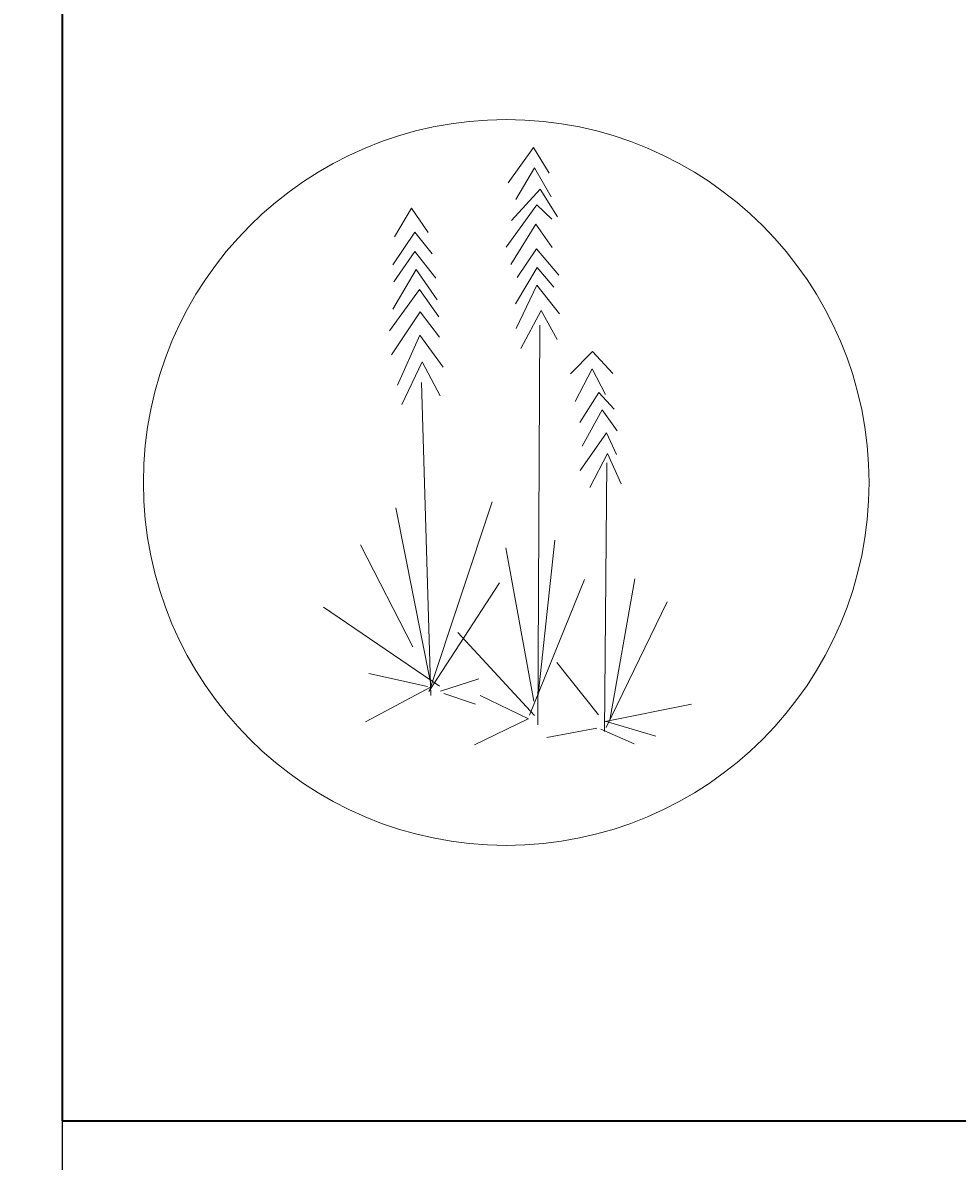
# Model space of a CAD drawing. Units: inches. Extents: x 8049 to 8459, y 820 to 1350.
# Tile 3 of 25: x 8083 to 8102, y 853 to 877. Entities that reach past the tile are written whole.
import ezdxf

# ---------------------------------------------------------------- set-up
doc = ezdxf.new("R2010")
doc.units = ezdxf.units.IN
doc.header["$MEASUREMENT"] = 0
for name, color, linetype, lineweight in [('A-ANNO-DIMS', 2, 'Continuous', 18), ('C-SITE-WALL', 7, 'Continuous', 35), ('zelen', 69, 'Continuous', 13)]:
    doc.layers.add(name, color=color, linetype=linetype, lineweight=lineweight)
doc.styles.get("Standard").update_dxf_attribs({"font": 'arial.ttf'})
doc.dimstyles.get("Standard").update_dxf_attribs({"dimtxt": 0.18, "dimasz": 0.18, "dimexe": 0.18, "dimexo": 0.0625, "dimgap": 0.09, "dimtad": 0, "dimtih": 1, "dimtoh": 1, "dimdec": 4, "dimzin": 0, "dimdsep": 46, "dimtxsty": 'Standard', "dimcen": 0.09, "dimadec": 0, "dimazin": 0, "dimtfac": 1, "dimtdec": 4, "dimtofl": 0, "dimtmove": 0, "dimatfit": 3, "dimfxl": 1, "dimtolj": 1, "dimtzin": 0, "dimarcsym": 0})

# ---------------------------------------------------------------- blocks, each defined once
blk = doc.blocks.new('z_04')
for p, q in [((2.7, 414.9), (37.8, 463.9)), ((37.8, 463.9), (59.6, 428.2)), ((13.1, 392), (38.9, 435.6)), ((38.9, 435.6), (62.3, 395.4)), ((7.3, 362.9), (46.8, 406.2)), ((46.8, 406.2), (71, 367.7)), ((-154.8, 340), (-131.1, 379.6)), ((-131.1, 379.6), (-108, 346.2)), ((0, 325.8), (42.4, 384.4)), ((42.4, 384.4), (63.1, 364.6)), ((6.3, 301.8), (40.8, 357.5)), ((40.8, 357.5), (63.6, 325.5)), ((-157.2, 301.5), (-126.5, 346.8)), ((-126.5, 346.8), (-102.5, 316.5)), ((-155.9, 278), (-126.5, 319.9)), ((-126.5, 319.9), (-97.4, 282.8)), ((15.2, 283.7), (41.9, 323.3)), ((41.9, 323.3), (72.9, 287.1)), ((-156.9, 239.8), (-124.6, 295)), ((-124.6, 295), (-95.5, 253.1)), ((12.8, 247.5), (42.7, 297.5)), ((42.7, 297.5), (66.1, 270.4)), ((13.9, 213), (42.2, 273.2)), ((42.2, 273.2), (73.7, 233.6)), ((-161.6, 209.9), (-120.2, 267)), ((-120.2, 267), (-93.3, 229.4)), ((20.4, 185.3), (48.4, 238.1)), ((48.4, 238.1), (70.4, 198)), ((-159.1, 176.8), (-119.4, 236.5)), ((-119.4, 236.5), (-92.5, 201.1)), ((43.8, -335.7), (46.5, 217.8)), ((-150.7, 134.9), (-119.7, 203.9)), ((-119.7, 203.9), (-87.6, 159.8)), ((89.2, 150.5), (119.4, 181.3)), ((119.4, 181.3), (147.7, 150.8)), ((-144.4, 107.8), (-116.4, 166.9)), ((-116.4, 166.9), (-91.4, 119.9)), ((95.5, 112), (119.1, 157.3)), ((119.1, 157.3), (137.6, 121.6)), ((-104.4, -294.9), (-117.5, 138.6)), ((102, 82.9), (128.4, 124.4)), ((128.4, 124.4), (149.3, 101.5)), ((105, 50.3), (132.7, 100.7)), ((132.7, 100.7), (153.7, 71.6)), ((102.5, 16.7), (138.7, 68.7)), ((138.7, 68.7), (152.6, 38.5)), ((115.6, -6.8), (140.1, 40.2)), ((140.1, 40.2), (159.1, -2)), ((136, -344.8), (139.5, 27.2)), ((-106.6, -289.6), (-19.3, -26.6)), ((-105, -276.9), (-153.1, -35.1)), ((-129.5, -227.7), (-202.1, -86.3)), ((38.1, -302.9), (-0.8, -90.5)), ((44.1, -294.7), (67.5, -80)), ((-107.2, -289.3), (-9.5, -139.2)), ((32.4, -322.2), (108.5, -134.3)), ((143.3, -329.2), (178.2, -133.5)), ((-92.5, -282), (-253, -172.8)), ((138.4, -339.1), (223, -165.2)), ((38.9, -322.7), (-67.2, -207.9)), ((127.8, -321.9), (69.9, -249.5)), ((-109.3, -282.6), (-190.4, -264.7)), ((-104.2, -282.8), (-195, -331.5)), ((-91.1, -288.8), (-37.8, -272.1)), ((-86.5, -292.2), (-42.7, -306.9)), ((31, -327.5), (-36.2, -295)), ((136.8, -330.9), (256.5, -306.9)), ((30.5, -327.5), (-44.1, -363.4)), ((137.1, -330.6), (207, -351.3)), ((125.4, -340), (56.3, -353.3)), ((131.1, -341.7), (177.3, -361.8))]:
    blk.add_line(p, q)
blk.add_circle((0, 0), 502.5)
blk = doc.blocks.new('*D50')
at = {"layer": 'A-ANNO-DIMS', "color": 0, "lineweight": -2, "transparency": 16777216}
for p, q in [((8083.335, 1045.871), (8049.617, 1045.871)), ((8049.797, 1045.691), (8049.797, 945.553)), ((8049.797, 845.051), (8049.797, 945.189)), ((8074.335, 844.871), (8049.617, 844.871))]:
    blk.add_line(p, q, dxfattribs=at)
at = {"layer": 'A-ANNO-DIMS', "color": 0, "transparency": 16777216}
for points in [[(8049.767, 1045.691), (8049.827, 1045.691), (8049.797, 1045.871)], [(8049.767, 845.051), (8049.827, 845.051), (8049.797, 844.871)]]:
    blk.add_solid(points, dxfattribs=at)
at = {"layer": 'Defpoints', "color": 0, "transparency": 16777216}
for p in [(8049.797, 1045.871), (8083.397, 1045.871), (8074.397, 844.871)]:
    blk.add_point(p, dxfattribs=at)
at = {"layer": 'A-ANNO-DIMS', "color": 0, "transparency": 16777216, "insert": (8049.797, 945.371), "char_height": 0.18, "attachment_point": 5}
blk.add_mtext('\\A1;201', dxfattribs=at)
blk = doc.blocks.new('*D70')
at = {"layer": 'A-ANNO-DIMS', "color": 0, "lineweight": -2, "transparency": 16777216}
for p, q in [((8083.397, 1045.808), (8083.397, 820.091)), ((8137.397, 1045.808), (8137.397, 820.091)), ((8083.577, 820.271), (8110.179, 820.271)), ((8137.217, 820.271), (8110.616, 820.271))]:
    blk.add_line(p, q, dxfattribs=at)
at = {"layer": 'A-ANNO-DIMS', "color": 0, "transparency": 16777216}
for points in [[(8083.577, 820.301), (8083.577, 820.241), (8083.397, 820.271)], [(8137.217, 820.301), (8137.217, 820.241), (8137.397, 820.271)]]:
    blk.add_solid(points, dxfattribs=at)
at = {"layer": 'Defpoints', "color": 0, "transparency": 16777216}
for p in [(8083.397, 1045.871), (8137.397, 1045.871), (8083.397, 820.271)]:
    blk.add_point(p, dxfattribs=at)
at = {"layer": 'A-ANNO-DIMS', "color": 0, "transparency": 16777216, "insert": (8110.397, 820.271), "char_height": 0.18, "attachment_point": 5}
blk.add_mtext('\\A1;54', dxfattribs=at)
blk = doc.blocks.new('*D76')
at = {"layer": 'A-ANNO-DIMS', "color": 0, "lineweight": -2, "transparency": 16777216}
for p, q in [((8083.397, 1054.808), (8083.397, 820.091)), ((8299.397, 1054.808), (8299.397, 820.091)), ((8083.577, 820.271), (8191.107, 820.271)), ((8299.217, 820.271), (8191.688, 820.271))]:
    blk.add_line(p, q, dxfattribs=at)
at = {"layer": 'A-ANNO-DIMS', "color": 0, "transparency": 16777216}
for points in [[(8083.577, 820.301), (8083.577, 820.241), (8083.397, 820.271)], [(8299.217, 820.301), (8299.217, 820.241), (8299.397, 820.271)]]:
    blk.add_solid(points, dxfattribs=at)
at = {"layer": 'Defpoints', "color": 0, "transparency": 16777216}
for p in [(8083.397, 1054.871), (8299.397, 1054.871), (8299.397, 820.271)]:
    blk.add_point(p, dxfattribs=at)
at = {"layer": 'A-ANNO-DIMS', "color": 0, "transparency": 16777216, "insert": (8191.397, 820.271), "char_height": 0.18, "attachment_point": 5}
blk.add_mtext('\\A1;216', dxfattribs=at)
blk = doc.blocks.new('*D88')
at = {"layer": 'A-ANNO-DIMS', "color": 0, "lineweight": -2, "transparency": 16777216}
for p, q in [((8083.397, 1162.808), (8083.397, 820.091)), ((8139.397, 1162.808), (8139.397, 820.091)), ((8083.577, 820.271), (8111.179, 820.271)), ((8139.217, 820.271), (8111.616, 820.271))]:
    blk.add_line(p, q, dxfattribs=at)
at = {"layer": 'A-ANNO-DIMS', "color": 0, "transparency": 16777216}
for points in [[(8083.577, 820.301), (8083.577, 820.241), (8083.397, 820.271)], [(8139.217, 820.301), (8139.217, 820.241), (8139.397, 820.271)]]:
    blk.add_solid(points, dxfattribs=at)
at = {"layer": 'Defpoints', "color": 0, "transparency": 16777216}
for p in [(8083.397, 1162.871), (8139.397, 1162.871), (8139.397, 820.271)]:
    blk.add_point(p, dxfattribs=at)
at = {"layer": 'A-ANNO-DIMS', "color": 0, "transparency": 16777216, "insert": (8111.397, 820.271), "char_height": 0.18, "attachment_point": 5}
blk.add_mtext('\\A1;56', dxfattribs=at)

msp = doc.modelspace()

# ---------------------------------------------------------------- linework, layer by layer
at = {"layer": 'C-SITE-WALL'}
for p, q in [((8083.3974, 1315.8706), (8083.3974, 853.8706)), ((8083.3974, 853.8706), (8219.8974, 853.8706))]:
    msp.add_line(p, q, dxfattribs=at)

# ---------------------------------------------------------------- block references
at = {"layer": 'zelen', "xscale": 0.0151365556588967, "yscale": 0.0151365556588967, "zscale": 0.0151365556588967}
msp.add_blockref('z_04', (8092.7087, 867.2506), dxfattribs=at)

# ---------------------------------------------------------------- dimensions: what is measured, and where the dimension line sits
at = {"layer": 'A-ANNO-DIMS'}
for base, p1, p2, picture, middle in [((8139.3974, 820.2706), (8083.3974, 1162.8706), (8139.3974, 1162.8706), '*D88', (8111.3974, 820.2706)), ((8299.3974, 820.2706), (8083.3974, 1054.8706), (8299.3974, 1054.8706), '*D76', (8191.3974, 820.2706)), ((8083.3974, 820.2706), (8137.3974, 1045.8706), (8083.3974, 1045.8706), '*D70', (8110.3974, 820.2706))]:
    dim = msp.add_linear_dim(base=base, p1=p1, p2=p2, dimstyle='Standard', override={"dimdec": 0, "dimlfac": 1, "dimrnd": 0, "dimzin": 0, "dimdsep": 46, "dimlunit": 2}, dxfattribs=at)
    dim.commit()
    dim.dimension.update_dxf_attribs({"geometry": picture, "text_midpoint": middle})
dim = msp.add_linear_dim(base=(8049.7974, 1045.8706), p1=(8074.3974, 844.8706), p2=(8083.3974, 1045.8706), angle=90, dimstyle='Standard', override={"dimdec": 0, "dimlfac": 1, "dimrnd": 0, "dimzin": 0, "dimdsep": 46, "dimlunit": 2}, dxfattribs=at)
dim.commit()
dim.dimension.update_dxf_attribs({"geometry": '*D50', "text_midpoint": (8049.7974, 945.3706)})

doc.saveas('drawing.dxf')
